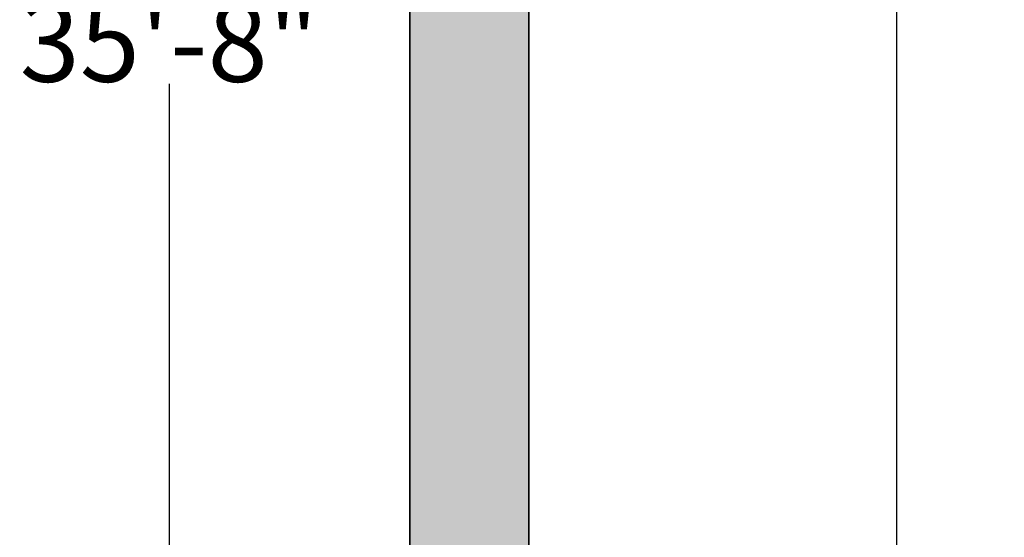
# Model space of a CAD drawing. Units: inches. Extents: x -15 to 423, y -713 to 71.
# Tile 3 of 24: x -4 to 70, y -234 to -195. Entities that reach past the tile are written whole.
import ezdxf

# ---------------------------------------------------------------- set-up
doc = ezdxf.new("R2010")
doc.units = ezdxf.units.IN
doc.header["$MEASUREMENT"] = 0
for name, color, linetype, lineweight in [('A-ANNO-DIMS', 2, 'Continuous', 18), ('A-WALL', 7, 'Continuous', 35), ('A-WALL-PATT', 8, 'Continuous', 13)]:
    doc.layers.add(name, color=color, linetype=linetype, lineweight=lineweight)
doc.styles.get("Standard").update_dxf_attribs({"font": 'arial.ttf'})
doc.dimstyles.get("Standard").update_dxf_attribs({"dimtxt": 0.18, "dimasz": 0.18, "dimexe": 0.18, "dimexo": 0.0625, "dimgap": 0.09, "dimtad": 0, "dimtih": 1, "dimtoh": 1, "dimdec": 0, "dimzin": 0, "dimdsep": 46, "dimlunit": 3, "dimtxsty": 'Standard', "dimcen": 0.09, "dimadec": 0, "dimazin": 0, "dimtfac": 1, "dimtdec": 0, "dimtofl": 0, "dimtmove": 0, "dimatfit": 3, "dimfxl": 1, "dimtolj": 1, "dimtzin": 0, "dimarcsym": 0})

# ---------------------------------------------------------------- blocks, each defined once
blk = doc.blocks.new('*D8')
at = {"layer": 'A-ANNO-DIMS', "color": 0, "lineweight": -2, "transparency": 16777216}
for p, q in [((25.018, 17.5), (6.724, 17.5)), ((6.904, 17.32), (6.904, -193.094)), ((6.904, -409.82), (6.904, -199.405)), ((34.018, -410), (6.724, -410))]:
    blk.add_line(p, q, dxfattribs=at)
at = {"layer": 'A-ANNO-DIMS', "color": 0, "transparency": 16777216}
for points in [[(6.874, 17.32), (6.934, 17.32), (6.904, 17.5)], [(6.874, -409.82), (6.934, -409.82), (6.904, -410)]]:
    blk.add_solid(points, dxfattribs=at)
at = {"layer": 'Defpoints', "color": 0, "transparency": 16777216}
for p in [(25.081, 17.5), (6.904, -410), (34.081, -410)]:
    blk.add_point(p, dxfattribs=at)
at = {"layer": 'A-ANNO-DIMS', "color": 0, "transparency": 16777216, "insert": (6.904, -196.25), "char_height": 6, "attachment_point": 5}
blk.add_mtext('\\A1;35\'-8"', dxfattribs=at)
blk = doc.blocks.new('*D37')
at = {"layer": 'A-ANNO-DIMS', "color": 0, "lineweight": -2, "transparency": 16777216}
for p, q in [((34.081, -396.437), (34.081, 57.43)), ((61.878, -396.437), (61.878, 57.43)), ((34.261, 57.25), (47.648, 57.25)), ((61.698, 57.25), (48.31, 57.25))]:
    blk.add_line(p, q, dxfattribs=at)
at = {"layer": 'A-ANNO-DIMS', "color": 0, "transparency": 16777216}
for points in [[(34.261, 57.28), (34.261, 57.22), (34.081, 57.25)], [(61.698, 57.28), (61.698, 57.22), (61.878, 57.25)]]:
    blk.add_solid(points, dxfattribs=at)
at = {"layer": 'Defpoints', "color": 0, "transparency": 16777216}
for p in [(61.878, 57.25), (34.081, -396.5), (61.878, -396.5)]:
    blk.add_point(p, dxfattribs=at)
at = {"layer": 'A-ANNO-DIMS', "color": 0, "transparency": 16777216, "insert": (47.979, 57.25), "char_height": 0.18, "attachment_point": 5}
blk.add_mtext('\\A1;2\'-4"', dxfattribs=at)

msp = doc.modelspace()

# ---------------------------------------------------------------- hatches: boundary and pattern name
at = {"layer": 'A-WALL-PATT'}
h = msp.add_hatch(color=256, dxfattribs=at)
h.dxf.hatch_style = 1
h.paths.add_polyline_path([(34.081, -349.58), (25.081, -349.58), (25.081, -431), (34.081, -431)])
h.paths.add_polyline_path([(34.081, -467), (25.081, -467), (25.081, -673), (34.081, -673)])
h.paths.add_polyline_path([(373.081, -668.5), (182.081, -668.5), (182.081, -673), (373.081, -673)])
h.paths.add_polyline_path([(253.199, -597.5), (191.081, -597.5), (191.081, -594.5), (182.081, -594.5), (182.081, -606.5), (253.199, -606.5)])
h.paths.add_polyline_path([(373.081, -597.5), (313.199, -597.5), (313.199, -606.5), (373.081, -606.5)])
h.paths.add_polyline_path([(382.081, -545.549), (373.081, -545.549), (373.081, -673), (382.081, -673)])
h.paths.add_polyline_path([(139.081, -488), (34.081, -488), (34.081, -497), (139.081, -497), (139.081, -492.5)])
h.paths.add_polyline_path([(139.081, -396.5), (128.581, -396.5), (128.581, -352.79), (124.081, -352.79), (124.081, -396.5), (34.081, -396.5), (34.081, -410), (139.081, -410), (139.081, -403.25)])
h.paths.add_polyline_path([(191.081, -396.5), (179.081, -396.5), (179.081, -410), (182.081, -410), (182.081, -488), (179.081, -488), (179.081, -497), (182.081, -497), (182.081, -501.431), (191.081, -501.431)])
h.paths.add_polyline_path([(373.081, -396.5), (253.081, -396.5), (253.081, -393.5), (248.581, -393.5), (248.581, -401), (284.581, -401), (284.581, -404), (289.081, -404), (289.081, -401), (373.081, -401)])
h.paths.add_polyline_path([(373.081, -449), (289.081, -449), (289.081, -432), (286.831, -432), (284.581, -432), (284.581, -453.5), (373.081, -453.5)])
h.paths.add_polyline_path([(382.081, -344.267), (373.081, -344.267), (373.081, -413.683), (382.081, -413.683)])
h.paths.add_polyline_path([(382.081, -437.683), (373.081, -437.683), (373.081, -485.549), (382.081, -485.549)])
h.paths.add_polyline_path([(34.081, -188.264), (25.081, -188.264), (25.081, -289.58), (34.081, -289.58)])
h.paths.add_polyline_path([(164.081, -236), (34.081, -236), (34.081, -240.5), (124.081, -240.5), (124.081, -293.122), (128.581, -293.122), (128.581, -240.5), (164.081, -240.5), (164.081, -238.25)])
h.paths.add_polyline_path([(373.081, -236), (242.581, -236), (242.581, -238.25), (242.581, -240.5), (248.581, -240.5), (248.581, -353.5), (250.831, -353.5), (253.081, -353.5), (253.081, -240.5), (373.081, -240.5)])
h.paths.add_polyline_path([(382.081, -190.86), (373.081, -190.86), (373.081, -284.267), (382.081, -284.267)])
h.paths.add_polyline_path([(211.581, -80), (253.581, -80), (253.581, -77.75), (253.581, -75.5), (153.581, -75.5), (153.581, -77.75), (153.581, -80), (207.081, -80), (207.081, -236), (204.081, -236), (204.081, -240.5), (214.581, -240.5), (214.581, -236), (211.581, -236)])
h.paths.add_polyline_path([(34.081, 8.5), (70.358, 8.5), (70.358, 17.5), (25.081, 17.5), (25.081, -128.264), (34.081, -128.264)])
h.paths.add_polyline_path([(110.581, 17.5), (94.358, 17.5), (94.358, 8.5), (110.581, 8.5)])
h.paths.add_polyline_path([(296.581, 17.5), (110.581, 17.5), (110.581, 13), (296.581, 13)])
h.paths.add_polyline_path([(110.581, 8.5), (106.081, 8.5), (106.081, -75.5), (103.081, -75.5), (103.081, -80), (113.581, -80), (113.581, -77.75), (113.581, -75.5), (110.581, -75.5)])
h.paths.add_polyline_path([(75.081, -75.5), (34.081, -75.5), (34.081, -80), (75.081, -80), (75.081, -77.75)])
h.paths.add_polyline_path([(343.093, 17.5), (296.581, 17.5), (296.581, 13), (296.581, 8.5), (343.093, 8.5)])
h.paths.add_polyline_path([(304.081, -75.5), (301.081, -75.5), (301.081, 8.5), (296.581, 8.5), (296.581, -75.5), (293.581, -75.5), (293.581, -80), (304.081, -80)])
h.paths.add_polyline_path([(382.081, 17.5), (367.093, 17.5), (367.093, 8.5), (373.081, 8.5), (373.081, -130.86), (382.081, -130.86)])
h.paths.add_polyline_path([(373.081, -75.5), (332.081, -75.5), (332.081, -77.75), (332.081, -80), (373.081, -80)])

# ---------------------------------------------------------------- linework, layer by layer
at = {"layer": 'A-WALL'}
for p, q in [((25.081, 17.5), (25.081, -673)), ((34.081, 8.5), (34.081, -673))]:
    msp.add_line(p, q, dxfattribs=at)

# ---------------------------------------------------------------- dimensions: what is measured, and where the dimension line sits
at = {"layer": 'A-ANNO-DIMS'}
dim = msp.add_linear_dim(base=(61.878, 57.25), p1=(34.081, -396.5), p2=(61.878, -396.5), dimstyle='Standard', override={"dimdec": 1, "dimlfac": 1, "dimrnd": 0, "dimzin": 1, "dimdsep": 46, "dimlunit": 4, "dimfrac": 2}, dxfattribs=at)
dim.commit()
dim.dimension.update_dxf_attribs({"geometry": '*D37', "text_midpoint": (47.979, 57.25)})
dim = msp.add_linear_dim(base=(6.904132698, -409.999899363), p1=(25.080555734, 17.500100637), p2=(34.080555734, -409.999899363), angle=90, dimstyle='Standard', override={"dimtxt": 6, "dimclrd": 0, "dimclre": 0, "dimclrt": 0}, dxfattribs=at)
dim.commit()
dim.dimension.update_dxf_attribs({"geometry": '*D8', "text_midpoint": (6.904132698, -196.249899363)})

doc.saveas('drawing.dxf')
